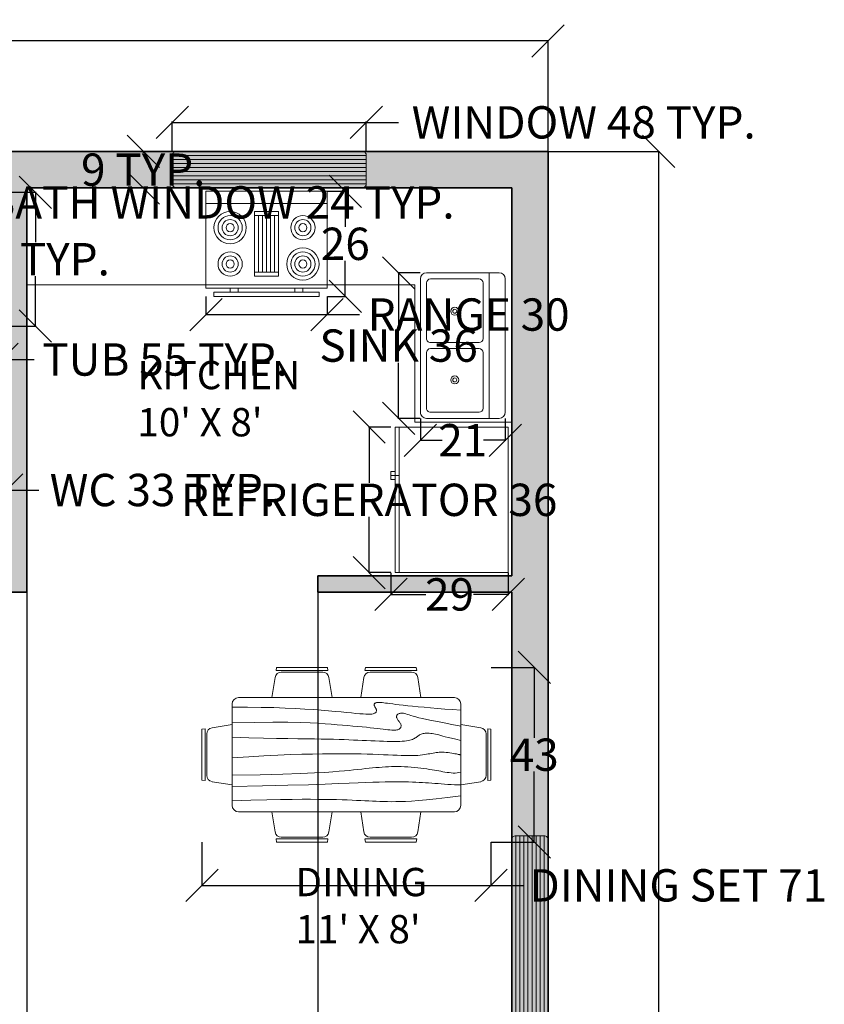
# Model space of a CAD drawing. Units: inches. Extents: x -8 to 447, y -560 to 47.
# Tile 5 of 5: x 248 to 447, y -196 to 47. Entities that reach past the tile are written whole.
import ezdxf

# ---------------------------------------------------------------- set-up
doc = ezdxf.new("R2010")
doc.units = ezdxf.units.IN
doc.header["$MEASUREMENT"] = 0
for name, color, linetype, lineweight in [('A-ANNO-DIMS', 2, 'Continuous', 18), ('A-AREA-IDEN', 7, 'Continuous', 18), ('A-EQPM', 9, 'Continuous', 18), ('A-FLOR-CASE', 8, 'Continuous', 18), ('A-FLOR-FIXT', 8, 'Continuous', 18), ('A-FURN', 8, 'Continuous', 18), ('A-WALL', 7, 'Continuous', 35), ('A-WALL-PATT', 251, 'Continuous', 13), ('WINDOW', 151, 'Continuous', 13)]:
    doc.layers.add(name, color=color, linetype=linetype, lineweight=lineweight)
doc.styles.get("Standard").update_dxf_attribs({"font": 'arial.ttf'})
doc.dimstyles.get("Standard").update_dxf_attribs({"dimtxt": 8, "dimasz": 8, "dimexe": 0.18, "dimexo": 0.0625, "dimgap": 0.09, "dimtad": 0, "dimtih": 1, "dimtoh": 1, "dimdec": 0, "dimzin": 0, "dimdsep": 46, "dimlunit": 4, "dimtxsty": 'Standard', "dimblk": 'OBLIQUE', "dimcen": 0.09, "dimadec": 0, "dimazin": 0, "dimtfac": 1, "dimtdec": 0, "dimtofl": 0, "dimtmove": 0, "dimatfit": 3, "dimldrblk": 'OBLIQUE', "dimfxl": 1, "dimtolj": 1, "dimtzin": 0, "dimarcsym": 0})

# ---------------------------------------------------------------- blocks, each defined once
blk = doc.blocks.new('WINDOW')
for p, q in [((0, -1.63), (48, -1.63)), ((0, -2.63), (48, -2.63)), ((0, -3.63), (48, -3.63)), ((0, -4.63), (48, -4.63)), ((0, -5.63), (48, -5.63)), ((0, -6.63), (48, -6.63)), ((0, -7.63), (48, -7.63)), ((0, -8.63), (48, -8.63))]:
    blk.add_line(p, q)
blk.add_lwpolyline([(48, -1.63), (48, -8.63, -0.414214), (47, -9.63), (1, -9.63, -0.414214), (0, -8.63), (0, -1.63, -0.414214), (1, -0.63), (47, -0.63, -0.414214)], format="xyb", close=True)
blk = doc.blocks.new('Dining Set - 36 x 72 in.')
for p, q in [((-22, 27.5), (-22.16, 26.5)), ((-5.84, 26.5), (-22.15, 26.5)), ((-22, 27.5), (-6, 27.5)), ((-20.52, 26), (-7.48, 26)), ((-5.84, 26.5), (-6, 27.5)), ((6, 27.5), (5.84, 26.5)), ((22.16, 26.5), (5.85, 26.5)), ((6, 27.5), (22, 27.5)), ((7.48, 26), (20.52, 26)), ((22.16, 26.5), (22, 27.5)), ((-22.5, 24.31), (-23.48, 18)), ((-4.52, 18), (-5.5, 24.31)), ((5.5, 24.31), (4.52, 18)), ((23.48, 18), (22.5, 24.31)), ((-36, 16), (-36, -16)), ((34, 18), (-34, 18)), ((36, -16), (36, 16)), ((-42.31, 8.5), (-36, 9.48)), ((42.31, 8.5), (36, 9.48)), ((-45.5, 8), (-44.5, 8.16)), ((-45.5, 8), (-45.5, -8)), ((-44.5, -8.16), (-44.5, 8.15)), ((-44, 6.52), (-44, -6.52)), ((44, 6.52), (44, -6.52)), ((45.5, 8), (44.5, 8.16)), ((44.5, -8.16), (44.5, 8.15)), ((45.5, 8), (45.5, -8)), ((-44.5, -8.16), (-45.5, -8)), ((-36, -9.48), (-42.31, -8.5)), ((36, -9.48), (42.31, -8.5)), ((44.5, -8.16), (45.5, -8)), ((-34, -18), (34, -18)), ((-22.5, -24.31), (-23.48, -18)), ((-4.52, -18), (-5.5, -24.31)), ((5.5, -24.31), (4.52, -18)), ((23.48, -18), (22.5, -24.31)), ((-22, -27.5), (-22.16, -26.5)), ((-5.84, -26.5), (-22.15, -26.5)), ((-22, -27.5), (-6, -27.5)), ((-20.52, -26), (-7.48, -26)), ((-5.84, -26.5), (-6, -27.5)), ((6, -27.5), (5.84, -26.5)), ((22.16, -26.5), (5.85, -26.5)), ((6, -27.5), (22, -27.5)), ((7.48, -26), (20.52, -26)), ((22.16, -26.5), (22, -27.5))]:
    blk.add_line(p, q)
for points in [[(-36, 15), (-31.18, 14.98), (-26.81, 14.91), (-22.85, 14.82), (-19.28, 14.69), (-16.04, 14.54), (-13.1, 14.37), (-10.42, 14.19), (-7.96, 14), (-5.69, 13.81), (-3.6, 13.63), (-1.7, 13.46), (0.04, 13.29), (1.59, 13.14), (2.98, 13.02), (4.2, 12.91), (5.25, 12.83), (6.14, 12.79), (6.88, 12.77), (7.49, 12.78), (7.98, 12.81), (8.37, 12.87), (8.67, 12.95), (8.9, 13.05), (9.08, 13.17), (9.22, 13.3), (9.32, 13.44), (9.39, 13.6), (9.43, 13.76), (9.44, 13.93), (9.42, 14.09), (9.39, 14.26), (9.33, 14.42), (9.26, 14.57), (9.18, 14.71), (9.1, 14.85), (9.01, 14.99), (8.93, 15.12), (8.85, 15.25), (8.79, 15.37), (8.75, 15.5), (8.73, 15.62), (8.73, 15.75), (8.76, 15.87), (8.81, 15.98), (8.89, 16.08), (8.98, 16.18), (9.11, 16.26), (9.25, 16.33), (9.42, 16.39), (9.62, 16.43), (9.85, 16.45), (10.12, 16.46), (10.45, 16.45), (10.82, 16.43), (11.25, 16.39), (11.75, 16.33), (12.32, 16.26), (12.97, 16.18), (13.72, 16.08), (14.57, 15.97), (15.54, 15.85), (16.64, 15.71), (17.89, 15.57), (19.29, 15.42), (20.86, 15.26), (22.59, 15.09), (24.47, 14.92), (26.51, 14.74), (28.68, 14.56), (30.99, 14.37), (33.43, 14.19), (36, 14)], [(-36, 10), (-28.98, 10.14), (-23.17, 10.2), (-18.42, 10.2), (-14.57, 10.14), (-11.44, 10.03), (-8.88, 9.89), (-6.72, 9.74), (-4.79, 9.58), (-2.97, 9.43), (-1.22, 9.29), (0.44, 9.15), (2.03, 9.01), (3.53, 8.88), (4.94, 8.75), (6.27, 8.63), (7.5, 8.5), (8.64, 8.38), (9.69, 8.25), (10.65, 8.14), (11.53, 8.03), (12.33, 7.94), (13.04, 7.86), (13.68, 7.79), (14.25, 7.75), (14.75, 7.73), (15.18, 7.73), (15.55, 7.76), (15.88, 7.8), (16.15, 7.87), (16.38, 7.95), (16.58, 8.05), (16.75, 8.17), (16.89, 8.3), (17.01, 8.45), (17.11, 8.6), (17.18, 8.77), (17.22, 8.95), (17.23, 9.13), (17.21, 9.31), (17.17, 9.5), (17.09, 9.69), (16.99, 9.88), (16.86, 10.06), (16.73, 10.25), (16.59, 10.44), (16.44, 10.62), (16.3, 10.81), (16.17, 11), (16.05, 11.19), (15.95, 11.37), (15.88, 11.56), (15.82, 11.74), (15.8, 11.92), (15.8, 12.09), (15.84, 12.26), (15.92, 12.42), (16.03, 12.57), (16.18, 12.71), (16.36, 12.83), (16.57, 12.94), (16.81, 13.02), (17.08, 13.07), (17.36, 13.1), (17.67, 13.08), (17.99, 13.03), (18.34, 12.95), (18.74, 12.83), (19.19, 12.68), (19.72, 12.51), (20.33, 12.32), (21.05, 12.1), (21.88, 11.88), (22.84, 11.63), (23.96, 11.37), (25.28, 11.09), (26.83, 10.77), (28.64, 10.4), (30.75, 9.99), (33.19, 9.53), (36, 9)], [(-36, 5.5), (-30.72, 5.33), (-26.07, 5.21), (-21.99, 5.12), (-18.43, 5.05), (-15.3, 5.01), (-12.55, 4.97), (-10.11, 4.95), (-7.92, 4.92), (-5.91, 4.88), (-4.06, 4.84), (-2.34, 4.79), (-0.74, 4.74), (0.77, 4.68), (2.22, 4.62), (3.62, 4.56), (5, 4.5), (6.37, 4.44), (7.73, 4.38), (9.07, 4.32), (10.38, 4.27), (11.63, 4.23), (12.83, 4.2), (13.96, 4.17), (15, 4.17), (15.95, 4.17), (16.82, 4.2), (17.6, 4.24), (18.3, 4.29), (18.93, 4.36), (19.49, 4.45), (19.98, 4.55), (20.42, 4.67), (20.8, 4.8), (21.13, 4.94), (21.42, 5.1), (21.69, 5.26), (21.93, 5.43), (22.15, 5.59), (22.37, 5.76), (22.58, 5.92), (22.81, 6.07), (23.04, 6.21), (23.29, 6.34), (23.55, 6.46), (23.84, 6.56), (24.14, 6.64), (24.47, 6.71), (24.83, 6.75), (25.22, 6.77), (25.64, 6.77), (26.09, 6.74), (26.55, 6.7), (27.04, 6.63), (27.54, 6.55), (28.06, 6.45), (28.58, 6.33), (29.12, 6.2), (29.71, 6.05), (30.37, 5.87), (31.14, 5.67), (32.05, 5.43), (33.14, 5.16), (34.45, 4.85), (36, 4.5)], [(-36, -1), (-30.79, -0.66), (-26.02, -0.38), (-21.65, -0.16), (-17.66, 0.01), (-14, 0.13), (-10.65, 0.21), (-7.58, 0.27), (-4.75, 0.29), (-2.13, 0.3), (0.29, 0.29), (2.53, 0.26), (4.61, 0.22), (6.55, 0.18), (8.36, 0.12), (10.06, 0.06), (11.67, 0), (13.19, -0.06), (14.63, -0.12), (16, -0.17), (17.28, -0.22), (18.48, -0.25), (19.6, -0.27), (20.63, -0.27), (21.58, -0.25), (22.45, -0.21), (23.24, -0.15), (23.95, -0.07), (24.61, 0.02), (25.22, 0.12), (25.79, 0.22), (26.32, 0.32), (26.83, 0.42), (27.33, 0.51), (27.81, 0.59), (28.29, 0.65), (28.77, 0.71), (29.26, 0.75), (29.76, 0.77), (30.29, 0.77), (30.83, 0.75), (31.41, 0.71), (32, 0.65), (32.59, 0.57), (33.16, 0.49), (33.7, 0.4), (34.19, 0.32), (34.62, 0.24), (34.96, 0.17), (35.21, 0.11), (35.38, 0.07), (35.5, 0.04), (35.59, 0.02), (35.66, 0.01), (35.74, 0), (35.84, 0), (36, 0)], [(-36, -6.5), (-27.18, -6.31), (-20.08, -6.13), (-14.47, -5.94), (-10.11, -5.76), (-6.78, -5.58), (-4.24, -5.41), (-2.26, -5.24), (-0.62, -5.08), (0.87, -4.93), (2.27, -4.79), (3.59, -4.65), (4.83, -4.52), (6, -4.4), (7.13, -4.29), (8.21, -4.18), (9.25, -4.08), (10.27, -3.99), (11.27, -3.91), (12.26, -3.85), (13.25, -3.79), (14.24, -3.75), (15.23, -3.73), (16.23, -3.73), (17.25, -3.75), (18.29, -3.79), (19.35, -3.86), (20.4, -3.94), (21.45, -4.03), (22.48, -4.14), (23.47, -4.25), (24.43, -4.38), (25.33, -4.5), (26.18, -4.62), (26.97, -4.75), (27.71, -4.87), (28.42, -4.99), (29.1, -5.11), (29.76, -5.23), (30.4, -5.35), (31.04, -5.46), (31.68, -5.56), (32.33, -5.66), (32.97, -5.73), (33.6, -5.78), (34.22, -5.78), (34.83, -5.75), (35.43, -5.65), (36, -5.5)], [(-36, -10), (-26.4, -9.81), (-18.47, -9.63), (-11.98, -9.45), (-6.74, -9.28), (-2.52, -9.12), (0.88, -8.98), (3.68, -8.85), (6.08, -8.75), (8.28, -8.67), (10.3, -8.61), (12.17, -8.57), (13.9, -8.54), (15.49, -8.53), (16.96, -8.54), (18.32, -8.56), (19.58, -8.58), (20.76, -8.62), (21.87, -8.66), (22.92, -8.71), (23.93, -8.77), (24.91, -8.83), (25.88, -8.89), (26.85, -8.97), (27.83, -9.04), (28.85, -9.12), (29.88, -9.2), (30.93, -9.28), (31.98, -9.35), (33.02, -9.41), (34.04, -9.46), (35.04, -9.49), (36, -9.5)], [(-36, -14.5), (-30.09, -14.34), (-25.03, -14.21), (-20.73, -14.13), (-17.08, -14.07), (-13.97, -14.05), (-11.3, -14.04), (-8.97, -14.06), (-6.88, -14.08), (-4.92, -14.12), (-3.09, -14.16), (-1.37, -14.21), (0.24, -14.26), (1.76, -14.32), (3.2, -14.38), (4.55, -14.44), (5.83, -14.5), (7.06, -14.56), (8.24, -14.62), (9.39, -14.68), (10.55, -14.72), (11.72, -14.76), (12.93, -14.79), (14.2, -14.8), (15.54, -14.79), (16.99, -14.76), (18.62, -14.71), (20.48, -14.6), (22.66, -14.44), (25.23, -14.22), (28.26, -13.91), (31.83, -13.51), (36, -13)]]:
    blk.add_lwpolyline(points)
for centre, start, end in [((-20.52, 24), 90, 171.1198), ((-7.48, 24), 8.881, 90), ((7.48, 24), 90, 171.1198), ((20.52, 24), 8.881, 90), ((-34, 16), 90, 180), ((34, 16), 0, 90), ((-42, 6.52), 98.8806, 180), ((42, 6.52), 0, 81.1194), ((-42, -6.52), 180, 261.1194), ((42, -6.52), 278.8806, 0), ((-34, -16), 180, 270), ((34, -16), 270, 0), ((-20.52, -24), 188.8802, 270), ((-7.48, -24), 270, 351.1191), ((7.48, -24), 188.8802, 270), ((20.52, -24), 270, 351.1191)]:
    blk.add_arc(centre, 2, start, end)
blk = doc.blocks.new('Range-Oven - 30 in top')
for p, q in [((0, -3), (30, -3)), ((12, -6), (18, -6)), ((13, -20), (13, -6)), ((14, -6), (14, -20)), ((15, -20), (15, -6)), ((16, -6), (16, -20)), ((17, -20), (17, -6)), ((18, -20), (12, -20)), ((6, -24), (6, -25)), ((8, -25), (8, -24)), ((22, -25), (22, -24)), ((24, -24), (24, -25))]:
    blk.add_line(p, q)
for points in [[(0, -24), (0, 0), (30, 0), (30, -24)], [(12, -21), (12, -5), (18, -5), (18, -21)], [(2, -26), (2, -25), (28, -25), (28, -26)]]:
    blk.add_lwpolyline(points, close=True)
for centre, radius in [((6, -9), 4), ((6, -9), 3), ((6, -9), 2), ((24, -9), 3), ((24, -9), 2), ((6, -9), 1), ((24, -9), 1), ((24, -18), 4), ((6, -18), 3), ((6, -18), 2), ((6, -18), 1), ((24, -18), 3), ((24, -18), 2), ((24, -18), 1)]:
    blk.add_circle(centre, radius)
blk = doc.blocks.new('Sink-double - 36 in top')
for p, q in [((-18, -4), (18, -4)), ((-0.75, -18.5), (-0.75, -6.5)), ((0.75, -6.5), (0.75, -18.5))]:
    blk.add_line(p, q)
for points in [[(-16.5, 0), (16.5, 0)], [(-18, -19.5), (-18, -1.5)], [(18, -1.5), (18, -19.5)], [(-16.5, -18.5), (-16.5, -6.5)], [(-15.5, -5.5), (-1.75, -5.5)], [(1.75, -5.5), (15.5, -5.5)], [(16.5, -6.5), (16.5, -18.5)], [(16.5, -21), (-16.5, -21)], [(-1.75, -19.5), (-15.5, -19.5)], [(15.5, -19.5), (1.75, -19.5)]]:
    blk.add_lwpolyline(points)
for centre, radius in [((-8.5, -12.5), 1), ((-8.5, -12.5), 0.5), ((8.5, -12.5), 1), ((8.5, -12.5), 0.5)]:
    blk.add_circle(centre, radius)
for centre, radius, start, end in [((-16.5, -1.5), 1.5, 90, 180), ((16.5, -1.5), 1.5, 0, 90), ((-15.5, -6.5), 1, 90, 180), ((-1.75, -6.5), 1, 0, 90), ((1.75, -6.5), 1, 90, 180), ((15.5, -6.5), 1, 0, 90), ((-15.5, -18.5), 1, 180, 270), ((-1.75, -18.5), 1, 270, 0), ((1.75, -18.5), 1, 180, 270), ((15.5, -18.5), 1, 270, 0), ((-16.5, -19.5), 1.5, 180, 270), ((16.5, -19.5), 1.5, 270, 0)]:
    blk.add_arc(centre, radius, start, end)
blk = doc.blocks.new('Refrigerator-2 door - 36 in top')
for p, q in [((0, -26.999999), (36, -26.999999)), ((11, -27.999999), (11, -28.999999)), ((11, -28.999999), (13, -28.999999)), ((12, -26.999999), (12, -28.999999)), ((13, -28.999999), (13, -27.999999))]:
    blk.add_line(p, q)
blk.add_lwpolyline([(0, -27.999999), (0, 0), (36, 0), (36, -27.999999)], close=True)
blk = doc.blocks.new('_Oblique')
at = {"color": 0, "linetype": 'ByBlock', "lineweight": -2}
blk.add_line((-0.5, -0.5), (0.5, 0.5), dxfattribs=at)
blk = doc.blocks.new('*D29')
at = {"layer": 'A-ANNO-DIMS', "color": 0, "lineweight": -2, "transparency": 16777216}
for p, q in [((285.7, 14.62), (285.7, 21.94)), ((333.7, 14.62), (333.7, 21.94)), ((285.7, 21.76), (333.7, 21.76)), ((333.7, 21.76), (341.7, 21.76))]:
    blk.add_line(p, q, dxfattribs=at)
at = {"layer": 'Defpoints', "color": 0, "transparency": 16777216}
for p in [(333.7, 21.76), (285.7, 14.56), (333.7, 14.56)]:
    blk.add_point(p, dxfattribs=at)
at = {"layer": 'A-ANNO-DIMS', "color": 0, "lineweight": -2, "transparency": 16777216, "xscale": 8, "yscale": 8, "zscale": 8, "rotation": 180}
blk.add_blockref('_Oblique', (285.7, 21.76), dxfattribs=at)
at = {"layer": 'A-ANNO-DIMS', "color": 0, "lineweight": -2, "transparency": 16777216, "xscale": 8, "yscale": 8, "zscale": 8}
blk.add_blockref('_Oblique', (333.7, 21.76), dxfattribs=at)
at = {"layer": 'A-ANNO-DIMS', "color": 0, "transparency": 16777216, "insert": (387.5, 21.76), "char_height": 8, "attachment_point": 5}
blk.add_mtext('\\A1;WINDOW 48 TYP.', dxfattribs=at)
blk = doc.blocks.new('*D30')
at = {"layer": 'A-ANNO-DIMS', "color": 0, "lineweight": -2, "transparency": 16777216}
for p, q in [((285.64, 14.56), (278.32, 14.56)), ((278.5, 14.56), (278.5, 14.23)), ((285.64, 5.56), (278.32, 5.56)), ((278.5, 5.56), (278.5, 5.89))]:
    blk.add_line(p, q, dxfattribs=at)
at = {"layer": 'Defpoints', "color": 0, "transparency": 16777216}
for p in [(278.5, 14.56), (285.7, 14.56), (285.7, 5.56)]:
    blk.add_point(p, dxfattribs=at)
at = {"layer": 'A-ANNO-DIMS', "color": 0, "lineweight": -2, "transparency": 16777216, "xscale": 8, "yscale": 8, "zscale": 8}
for p, rotation in [((278.5, 14.56), 90), ((278.5, 5.56), 270)]:
    blk.add_blockref('_Oblique', p, dxfattribs=dict(at, rotation=rotation))
at = {"layer": 'A-ANNO-DIMS', "color": 0, "transparency": 16777216, "insert": (278.5, 10.06), "char_height": 8, "attachment_point": 5}
blk.add_mtext('\\A1;9 TYP.', dxfattribs=at)
blk = doc.blocks.new('*D31')
at = {"layer": 'A-ANNO-DIMS', "color": 0, "lineweight": -2, "transparency": 16777216}
for p, q in [((203.7, 5.5), (203.7, 1.78)), ((227.7, 5.5), (227.7, 1.78)), ((203.7, 1.96), (227.7, 1.96)), ((227.7, 1.96), (235.7, 1.96))]:
    blk.add_line(p, q, dxfattribs=at)
at = {"layer": 'Defpoints', "color": 0, "transparency": 16777216}
for p in [(203.7, 5.56), (227.7, 5.56), (227.7, 1.96)]:
    blk.add_point(p, dxfattribs=at)
at = {"layer": 'A-ANNO-DIMS', "color": 0, "lineweight": -2, "transparency": 16777216, "xscale": 8, "yscale": 8, "zscale": 8, "rotation": 180}
blk.add_blockref('_Oblique', (203.7, 1.96), dxfattribs=at)
at = {"layer": 'A-ANNO-DIMS', "color": 0, "lineweight": -2, "transparency": 16777216, "xscale": 8, "yscale": 8, "zscale": 8}
blk.add_blockref('_Oblique', (227.7, 1.96), dxfattribs=at)
at = {"layer": 'A-ANNO-DIMS', "color": 0, "transparency": 16777216, "insert": (297.61, 1.96), "char_height": 8, "attachment_point": 5}
blk.add_mtext('\\A1;BATH WINDOW 24 TYP.', dxfattribs=at)
blk = doc.blocks.new('*D39')
at = {"layer": 'A-ANNO-DIMS', "color": 0, "lineweight": -2, "transparency": 16777216}
for p, q in [((211.63, -64.31), (211.63, -69.38)), ((244.67, -64.31), (244.67, -69.38)), ((211.63, -69.2), (244.67, -69.2)), ((244.67, -69.2), (252.67, -69.2))]:
    blk.add_line(p, q, dxfattribs=at)
at = {"layer": 'Defpoints', "color": 0, "transparency": 16777216}
for p in [(211.63, -64.25), (244.67, -64.25), (244.67, -69.2)]:
    blk.add_point(p, dxfattribs=at)
at = {"layer": 'A-ANNO-DIMS', "color": 0, "lineweight": -2, "transparency": 16777216, "xscale": 8, "yscale": 8, "zscale": 8, "rotation": 180}
blk.add_blockref('_Oblique', (211.63, -69.2), dxfattribs=at)
at = {"layer": 'A-ANNO-DIMS', "color": 0, "lineweight": -2, "transparency": 16777216, "xscale": 8, "yscale": 8, "zscale": 8}
blk.add_blockref('_Oblique', (244.67, -69.2), dxfattribs=at)
at = {"layer": 'A-ANNO-DIMS', "color": 0, "transparency": 16777216, "insert": (283.26, -69.2), "char_height": 8, "attachment_point": 5}
blk.add_mtext('\\A1;WC 33 TYP.', dxfattribs=at)
blk = doc.blocks.new('*D41')
at = {"layer": 'A-ANNO-DIMS', "color": 0, "lineweight": -2, "transparency": 16777216}
for p, q in [((188.4, -28.7), (188.4, -37.09)), ((243.54, -28.7), (243.54, -37.09)), ((188.4, -36.91), (243.54, -36.91)), ((243.54, -36.91), (251.54, -36.91))]:
    blk.add_line(p, q, dxfattribs=at)
at = {"layer": 'Defpoints', "color": 0, "transparency": 16777216}
for p in [(188.4, -28.64), (243.54, -28.64), (243.54, -36.91)]:
    blk.add_point(p, dxfattribs=at)
at = {"layer": 'A-ANNO-DIMS', "color": 0, "lineweight": -2, "transparency": 16777216, "xscale": 8, "yscale": 8, "zscale": 8, "rotation": 180}
blk.add_blockref('_Oblique', (188.4, -36.91), dxfattribs=at)
at = {"layer": 'A-ANNO-DIMS', "color": 0, "lineweight": -2, "transparency": 16777216, "xscale": 8, "yscale": 8, "zscale": 8}
blk.add_blockref('_Oblique', (243.54, -36.91), dxfattribs=at)
at = {"layer": 'A-ANNO-DIMS', "color": 0, "transparency": 16777216, "insert": (283.93, -36.91), "char_height": 8, "attachment_point": 5}
blk.add_mtext('\\A1;TUB 55 TYP.', dxfattribs=at)
blk = doc.blocks.new('*D42')
at = {"layer": 'A-ANNO-DIMS', "color": 0, "lineweight": -2, "transparency": 16777216}
for p, q in [((243.61, 4.45), (252, 4.45)), ((251.82, 4.45), (251.82, -7.92)), ((251.82, -28.64), (251.82, -16.28)), ((243.61, -28.64), (252, -28.64))]:
    blk.add_line(p, q, dxfattribs=at)
at = {"layer": 'Defpoints', "color": 0, "transparency": 16777216}
for p in [(243.54, 4.45), (251.82, 4.45), (243.54, -28.64)]:
    blk.add_point(p, dxfattribs=at)
at = {"layer": 'A-ANNO-DIMS', "color": 0, "lineweight": -2, "transparency": 16777216, "xscale": 8, "yscale": 8, "zscale": 8}
for p, rotation in [((251.82, 4.45), 90), ((251.82, -28.64), 270)]:
    blk.add_blockref('_Oblique', p, dxfattribs=dict(at, rotation=rotation))
at = {"layer": 'A-ANNO-DIMS', "color": 0, "transparency": 16777216, "insert": (251.82, -12.1), "char_height": 8, "attachment_point": 5}
blk.add_mtext('\\A1;33 TYP.', dxfattribs=at)
blk = doc.blocks.new('*D43')
at = {"layer": 'A-ANNO-DIMS', "color": 0, "lineweight": -2, "transparency": 16777216}
for p, q in [((293.04, -156.35), (293.04, -167.19)), ((364.53, -156.35), (364.53, -167.19)), ((293.04, -167.01), (364.53, -167.01)), ((364.53, -167.01), (372.53, -167.01))]:
    blk.add_line(p, q, dxfattribs=at)
at = {"layer": 'Defpoints', "color": 0, "transparency": 16777216}
for p in [(293.04, -156.29), (364.53, -156.29), (364.53, -167.01)]:
    blk.add_point(p, dxfattribs=at)
at = {"layer": 'A-ANNO-DIMS', "color": 0, "lineweight": -2, "transparency": 16777216, "xscale": 8, "yscale": 8, "zscale": 8, "rotation": 180}
blk.add_blockref('_Oblique', (293.04, -167.01), dxfattribs=at)
at = {"layer": 'A-ANNO-DIMS', "color": 0, "lineweight": -2, "transparency": 16777216, "xscale": 8, "yscale": 8, "zscale": 8}
blk.add_blockref('_Oblique', (364.53, -167.01), dxfattribs=at)
at = {"layer": 'A-ANNO-DIMS', "color": 0, "transparency": 16777216, "insert": (410.91, -167.01), "char_height": 8, "attachment_point": 5}
blk.add_mtext('\\A1;DINING SET 71', dxfattribs=at)
blk = doc.blocks.new('*D44')
at = {"layer": 'A-ANNO-DIMS', "color": 0, "lineweight": -2, "transparency": 16777216}
for p, q in [((364.59, -113.08), (375.44, -113.08)), ((375.26, -113.08), (375.26, -130.5)), ((375.26, -156.29), (375.26, -138.86)), ((364.59, -156.29), (375.44, -156.29))]:
    blk.add_line(p, q, dxfattribs=at)
at = {"layer": 'Defpoints', "color": 0, "transparency": 16777216}
for p in [(364.53, -113.08), (375.26, -113.08), (364.53, -156.29)]:
    blk.add_point(p, dxfattribs=at)
at = {"layer": 'A-ANNO-DIMS', "color": 0, "lineweight": -2, "transparency": 16777216, "xscale": 8, "yscale": 8, "zscale": 8}
for p, rotation in [((375.26, -113.08), 90), ((375.26, -156.29), 270)]:
    blk.add_blockref('_Oblique', p, dxfattribs=dict(at, rotation=rotation))
at = {"layer": 'A-ANNO-DIMS', "color": 0, "transparency": 16777216, "insert": (375.26, -134.68), "char_height": 8, "attachment_point": 5}
blk.add_mtext('\\A1;43', dxfattribs=at)
blk = doc.blocks.new('*D45')
at = {"layer": 'A-ANNO-DIMS', "color": 0, "lineweight": -2, "transparency": 16777216}
for p, q in [((294.01, -21.35), (294.01, -25.97)), ((324.01, -21.35), (324.01, -25.97)), ((294.01, -25.79), (324.01, -25.79)), ((324.01, -25.79), (332.01, -25.79))]:
    blk.add_line(p, q, dxfattribs=at)
at = {"layer": 'Defpoints', "color": 0, "transparency": 16777216}
for p in [(294.01, -21.29), (324.01, -21.29), (324.01, -25.79)]:
    blk.add_point(p, dxfattribs=at)
at = {"layer": 'A-ANNO-DIMS', "color": 0, "lineweight": -2, "transparency": 16777216, "xscale": 8, "yscale": 8, "zscale": 8, "rotation": 180}
blk.add_blockref('_Oblique', (294.01, -25.79), dxfattribs=at)
at = {"layer": 'A-ANNO-DIMS', "color": 0, "lineweight": -2, "transparency": 16777216, "xscale": 8, "yscale": 8, "zscale": 8}
blk.add_blockref('_Oblique', (324.01, -25.79), dxfattribs=at)
at = {"layer": 'A-ANNO-DIMS', "color": 0, "transparency": 16777216, "insert": (359.03, -25.79), "char_height": 8, "attachment_point": 5}
blk.add_mtext('\\A1;RANGE 30', dxfattribs=at)
blk = doc.blocks.new('*D46')
at = {"layer": 'A-ANNO-DIMS', "color": 0, "lineweight": -2, "transparency": 16777216}
for p, q in [((324.07, 4.71), (328.69, 4.71)), ((328.51, 4.71), (328.51, -4.11)), ((328.51, -21.29), (328.51, -12.46)), ((324.07, -21.29), (328.69, -21.29))]:
    blk.add_line(p, q, dxfattribs=at)
at = {"layer": 'Defpoints', "color": 0, "transparency": 16777216}
for p in [(324.01, 4.71), (328.51, 4.71), (324.01, -21.29)]:
    blk.add_point(p, dxfattribs=at)
at = {"layer": 'A-ANNO-DIMS', "color": 0, "lineweight": -2, "transparency": 16777216, "xscale": 8, "yscale": 8, "zscale": 8}
for p, rotation in [((328.51, 4.71), 90), ((328.51, -21.29), 270)]:
    blk.add_blockref('_Oblique', p, dxfattribs=dict(at, rotation=rotation))
at = {"layer": 'A-ANNO-DIMS', "color": 0, "transparency": 16777216, "insert": (328.51, -8.29), "char_height": 8, "attachment_point": 5}
blk.add_mtext('\\A1;26', dxfattribs=at)
blk = doc.blocks.new('*D47')
at = {"layer": 'A-ANNO-DIMS', "color": 0, "lineweight": -2, "transparency": 16777216}
for p, q in [((347.03, -15.47), (341.51, -15.47)), ((341.69, -15.47), (341.69, -29.24)), ((341.69, -51.47), (341.69, -37.7)), ((347.03, -51.47), (341.51, -51.47))]:
    blk.add_line(p, q, dxfattribs=at)
at = {"layer": 'Defpoints', "color": 0, "transparency": 16777216}
for p in [(347.09, -15.47), (341.69, -51.47), (347.09, -51.47)]:
    blk.add_point(p, dxfattribs=at)
at = {"layer": 'A-ANNO-DIMS', "color": 0, "lineweight": -2, "transparency": 16777216, "xscale": 8, "yscale": 8, "zscale": 8}
for p, rotation in [((341.69, -15.47), 90), ((341.69, -51.47), 270)]:
    blk.add_blockref('_Oblique', p, dxfattribs=dict(at, rotation=rotation))
at = {"layer": 'A-ANNO-DIMS', "color": 0, "transparency": 16777216, "insert": (341.69, -33.47), "char_height": 8, "attachment_point": 5}
blk.add_mtext('\\A1;SINK 36', dxfattribs=at)
blk = doc.blocks.new('*D48')
at = {"layer": 'A-ANNO-DIMS', "color": 0, "lineweight": -2, "transparency": 16777216}
for p, q in [((347.09, -51.53), (347.09, -57.05)), ((368.09, -51.53), (368.09, -57.05)), ((347.09, -56.87), (352.48, -56.87)), ((368.09, -56.87), (362.71, -56.87))]:
    blk.add_line(p, q, dxfattribs=at)
at = {"layer": 'Defpoints', "color": 0, "transparency": 16777216}
for p in [(347.09, -51.47), (368.09, -51.47), (368.09, -56.87)]:
    blk.add_point(p, dxfattribs=at)
at = {"layer": 'A-ANNO-DIMS', "color": 0, "lineweight": -2, "transparency": 16777216, "xscale": 8, "yscale": 8, "zscale": 8, "rotation": 180}
blk.add_blockref('_Oblique', (347.09, -56.87), dxfattribs=at)
at = {"layer": 'A-ANNO-DIMS', "color": 0, "lineweight": -2, "transparency": 16777216, "xscale": 8, "yscale": 8, "zscale": 8}
blk.add_blockref('_Oblique', (368.09, -56.87), dxfattribs=at)
at = {"layer": 'A-ANNO-DIMS', "color": 0, "transparency": 16777216, "insert": (357.59, -56.87), "char_height": 8, "attachment_point": 5}
blk.add_mtext('\\A1;21', dxfattribs=at)
blk = doc.blocks.new('*D49')
at = {"layer": 'A-ANNO-DIMS', "color": 0, "lineweight": -2, "transparency": 16777216}
for p, q in [((339.74, -53.63), (334.23, -53.63)), ((334.41, -53.63), (334.41, -67.4)), ((334.41, -89.63), (334.41, -75.86)), ((339.74, -89.63), (334.23, -89.63))]:
    blk.add_line(p, q, dxfattribs=at)
at = {"layer": 'Defpoints', "color": 0, "transparency": 16777216}
for p in [(339.81, -53.63), (334.41, -89.63), (339.81, -89.63)]:
    blk.add_point(p, dxfattribs=at)
at = {"layer": 'A-ANNO-DIMS', "color": 0, "lineweight": -2, "transparency": 16777216, "xscale": 8, "yscale": 8, "zscale": 8}
for p, rotation in [((334.41, -53.63), 90), ((334.41, -89.63), 270)]:
    blk.add_blockref('_Oblique', p, dxfattribs=dict(at, rotation=rotation))
at = {"layer": 'A-ANNO-DIMS', "color": 0, "transparency": 16777216, "insert": (334.41, -71.63), "char_height": 8, "attachment_point": 5}
blk.add_mtext('\\A1;REFRIGERATOR 36', dxfattribs=at)
blk = doc.blocks.new('*D50')
at = {"layer": 'A-ANNO-DIMS', "color": 0, "lineweight": -2, "transparency": 16777216}
for p, q in [((339.81, -89.69), (339.81, -95.21)), ((368.81, -89.69), (368.81, -95.21)), ((339.81, -95.03), (348.41, -95.03)), ((368.81, -95.03), (360.2, -95.03))]:
    blk.add_line(p, q, dxfattribs=at)
at = {"layer": 'Defpoints', "color": 0, "transparency": 16777216}
for p in [(339.81, -89.63), (368.81, -89.63), (368.81, -95.03)]:
    blk.add_point(p, dxfattribs=at)
at = {"layer": 'A-ANNO-DIMS', "color": 0, "lineweight": -2, "transparency": 16777216, "xscale": 8, "yscale": 8, "zscale": 8, "rotation": 180}
blk.add_blockref('_Oblique', (339.81, -95.03), dxfattribs=at)
at = {"layer": 'A-ANNO-DIMS', "color": 0, "lineweight": -2, "transparency": 16777216, "xscale": 8, "yscale": 8, "zscale": 8}
blk.add_blockref('_Oblique', (368.81, -95.03), dxfattribs=at)
at = {"layer": 'A-ANNO-DIMS', "color": 0, "transparency": 16777216, "insert": (354.31, -95.03), "char_height": 8, "attachment_point": 5}
blk.add_mtext('\\A1;29', dxfattribs=at)
blk = doc.blocks.new('*D51')
at = {"layer": 'A-ANNO-DIMS', "color": 0, "lineweight": -2, "transparency": 16777216}
for p, q in [((28.7, 14.62), (28.7, 42.09)), ((28.7, 41.91), (194.79, 41.91)), ((378.7, 41.91), (212.61, 41.91)), ((378.7, 14.62), (378.7, 42.09))]:
    blk.add_line(p, q, dxfattribs=at)
at = {"layer": 'Defpoints', "color": 0, "transparency": 16777216}
for p in [(378.7, 41.91), (28.7, 14.56), (378.7, 14.56)]:
    blk.add_point(p, dxfattribs=at)
at = {"layer": 'A-ANNO-DIMS', "color": 0, "lineweight": -2, "transparency": 16777216, "xscale": 8, "yscale": 8, "zscale": 8, "rotation": 180}
blk.add_blockref('_Oblique', (28.7, 41.91), dxfattribs=at)
at = {"layer": 'A-ANNO-DIMS', "color": 0, "lineweight": -2, "transparency": 16777216, "xscale": 8, "yscale": 8, "zscale": 8}
blk.add_blockref('_Oblique', (378.7, 41.91), dxfattribs=at)
at = {"layer": 'A-ANNO-DIMS', "color": 0, "transparency": 16777216, "insert": (203.7, 41.91), "char_height": 8, "attachment_point": 5}
blk.add_mtext('\\A1;350', dxfattribs=at)
blk = doc.blocks.new('*D52')
at = {"layer": 'A-ANNO-DIMS', "color": 0, "lineweight": -2, "transparency": 16777216}
for p, q in [((378.76, 14.56), (406.23, 14.56)), ((406.05, 14.56), (406.05, -252.27)), ((406.05, -527.44), (406.05, -260.61)), ((307.76, -527.44), (406.23, -527.44))]:
    blk.add_line(p, q, dxfattribs=at)
at = {"layer": 'Defpoints', "color": 0, "transparency": 16777216}
for p in [(378.7, 14.56), (307.7, -527.44), (406.05, -527.44)]:
    blk.add_point(p, dxfattribs=at)
at = {"layer": 'A-ANNO-DIMS', "color": 0, "lineweight": -2, "transparency": 16777216, "xscale": 8, "yscale": 8, "zscale": 8}
for p, rotation in [((406.05, 14.56), 90), ((406.05, -527.44), 270)]:
    blk.add_blockref('_Oblique', p, dxfattribs=dict(at, rotation=rotation))
at = {"layer": 'A-ANNO-DIMS', "color": 0, "transparency": 16777216, "insert": (406.05, -256.44), "char_height": 8, "attachment_point": 5}
blk.add_mtext('\\A1;542', dxfattribs=at)
blk = doc.blocks.new('*D63')
at = {"layer": 'A-ANNO-DIMS', "color": 0, "lineweight": -2, "transparency": 16777216}
for p, q in [((249.7, -94.5), (249.7, -554.97)), ((321.7, -94.5), (321.7, -554.97)), ((249.7, -554.79), (279.96, -554.79)), ((321.7, -554.79), (291.45, -554.79))]:
    blk.add_line(p, q, dxfattribs=at)
at = {"layer": 'Defpoints', "color": 0, "transparency": 16777216}
for p in [(249.7, -94.44), (321.7, -94.44), (321.7, -554.79)]:
    blk.add_point(p, dxfattribs=at)
at = {"layer": 'A-ANNO-DIMS', "color": 0, "lineweight": -2, "transparency": 16777216, "xscale": 8, "yscale": 8, "zscale": 8, "rotation": 180}
blk.add_blockref('_Oblique', (249.7, -554.79), dxfattribs=at)
at = {"layer": 'A-ANNO-DIMS', "color": 0, "lineweight": -2, "transparency": 16777216, "xscale": 8, "yscale": 8, "zscale": 8}
blk.add_blockref('_Oblique', (321.7, -554.79), dxfattribs=at)
at = {"layer": 'A-ANNO-DIMS', "color": 0, "transparency": 16777216, "insert": (285.7, -554.79), "char_height": 8, "attachment_point": 5}
blk.add_mtext('\\A1;72', dxfattribs=at)

msp = doc.modelspace()

# ---------------------------------------------------------------- hatches: boundary and pattern name
at = {"layer": 'A-WALL-PATT'}
h = msp.add_hatch(color=256, dxfattribs=at)
h.dxf.hatch_style = 1
h.paths.add_polyline_path([(378.702, 14.56), (333.702, 14.56), (333.702, 5.56), (369.702, 5.56), (369.702, -90.44), (321.702, -90.44), (321.702, -94.44), (369.702, -94.44), (369.702, -154.733), (378.702, -154.733)])
h.paths.add_polyline_path([(285.702, 14.56), (227.702, 14.56), (227.702, 5.56), (245.702, 5.56), (245.702, -90.44), (239.702, -90.44), (239.702, -94.44), (249.702, -94.44), (249.702, -90.44), (249.702, 5.56), (285.702, 5.56)])
h.paths.add_polyline_path([(203.702, 14.56), (133.702, 14.56), (133.702, 5.56), (181.702, 5.56), (181.702, -132.44), (175.702, -132.44), (175.702, -136.44), (185.702, -136.44), (185.702, -94.44), (209.702, -94.44), (209.702, -90.44), (185.702, -90.44), (185.702, 5.56), (203.702, 5.56)])
h = msp.add_hatch(color=256, dxfattribs=at)
h.dxf.hatch_style = 1
h.paths.add_polyline_path([(378.702, 14.56), (227.702, 14.56), (227.702, 5.56), (245.702, 5.56), (245.702, -90.44), (239.702, -90.44), (239.702, -94.44), (249.702, -94.44), (249.702, -90.44), (249.702, 5.56), (369.702, 5.56), (369.702, -90.44), (321.702, -90.44), (321.702, -94.44), (369.702, -94.44), (369.702, -452.44), (325.702, -452.44), (325.702, -456.44), (369.702, -456.44), (369.702, -500.44), (309.702, -500.44), (309.702, -509.44), (369.702, -509.44), (369.702, -525.44), (378.702, -525.44)])

# ---------------------------------------------------------------- linework, layer by layer
at = {"layer": 'A-FLOR-CASE'}
for p, q in [((249.702, -18.44), (345.702, -18.44)), ((345.702, -18.44), (345.702, -52.44)), ((345.702, -52.44), (345.702, -18.44)), ((345.702, -52.44), (369.702, -52.44))]:
    msp.add_line(p, q, dxfattribs=at)
at = {"layer": 'A-WALL'}
for p, q in [((28.702, 14.56), (378.702, 14.56)), ((378.702, 14.56), (378.702, -525.44)), ((249.702, 5.56), (369.702, 5.56)), ((249.702, -90.44), (249.702, 5.56)), ((369.702, 5.56), (369.702, -90.44)), ((369.702, -90.44), (369.702, 5.56)), ((249.702, -90.44), (249.702, -94.44)), ((321.702, -90.44), (369.702, -90.44)), ((321.702, -90.44), (321.702, -94.44)), ((239.702, -94.44), (249.702, -94.44)), ((321.702, -94.44), (369.702, -94.44)), ((369.702, -94.44), (369.702, -452.44))]:
    msp.add_line(p, q, dxfattribs=at)

# ---------------------------------------------------------------- block references
at = {"layer": 'A-EQPM'}
msp.add_blockref('Range-Oven - 30 in top', (294.008, 4.71), dxfattribs=at)
at = {"layer": 'A-EQPM', "rotation": 270}
msp.add_blockref('Refrigerator-2 door - 36 in top', (368.807, -53.63), dxfattribs=at)
at = {"layer": 'A-FLOR-FIXT', "rotation": 270}
msp.add_blockref('Sink-double - 36 in top', (368.095, -33.468), dxfattribs=at)
at = {"layer": 'A-FURN', "xscale": 0.7856607656645134, "yscale": 0.7856607656645134, "zscale": 0.7856607656645134}
msp.add_blockref('Dining Set - 36 x 72 in.', (328.784, -134.682), dxfattribs=at)
at = {"layer": 'WINDOW'}
msp.add_blockref('WINDOW', (285.702, 15.195), dxfattribs=at)
at = {"layer": 'WINDOW', "rotation": 270}
msp.add_blockref('WINDOW', (379.337, -154.733), dxfattribs=at)

# ---------------------------------------------------------------- texts
at = {"layer": 'A-AREA-IDEN', "char_height": 7, "attachment_point": 1}
for s, width, insert in [("KITCHEN\\P10' X 8'", 101.37701, (277.064, -37.257)), ("DINING\\P11' X 8'", 131.16623, (316.19, -162.691))]:
    msp.add_mtext_dynamic_manual_height_columns(s, width=width, gutter_width=1, heights=[0], dxfattribs=dict(at, insert=insert))

# ---------------------------------------------------------------- dimensions: what is measured, and where the dimension line sits
at = {"layer": 'A-ANNO-DIMS'}
for base, p1, p2, picture, middle in [((378.702, 41.91), (28.702, 14.56), (378.702, 14.56), '*D51', (203.702, 41.91)), ((368.095, -56.868), (347.095, -51.468), (368.095, -51.468), '*D48', (357.595, -56.868)), ((368.807, -95.03), (339.807, -89.63), (368.807, -89.63), '*D50', (354.307, -95.03)), ((321.702, -554.79), (249.702, -94.44), (321.702, -94.44), '*D63', (285.702, -554.79))]:
    dim = msp.add_linear_dim(base=base, p1=p1, p2=p2, dimstyle='Standard', override={"dimdec": 0, "dimlfac": 1, "dimrnd": 0, "dimzin": 0, "dimdsep": 46, "dimlunit": 2}, dxfattribs=at)
    dim.commit()
    dim.dimension.update_dxf_attribs({"geometry": picture, "text_midpoint": middle})
for base, p1, p2, text, picture, middle in [((333.702, 21.76), (285.702, 14.56), (333.702, 14.56), 'WINDOW <> TYP.', '*D29', (387.498, 21.76)), ((227.702, 1.96), (203.702, 5.56), (227.702, 5.56), 'BATH WINDOW <> TYP.', '*D31', (297.612, 1.96)), ((324.008, -25.79), (294.008, -21.29), (324.008, -21.29), 'RANGE <>', '*D45', (359.031, -25.79)), ((243.545, -36.914), (188.397, -28.642), (243.545, -28.642), 'TUB <> TYP.', '*D41', (283.935, -36.914)), ((244.672, -69.204), (211.626, -64.247), (244.672, -64.247), 'WC <> TYP.', '*D39', (283.258, -69.204)), ((364.532, -167.011), (293.037, -156.287), (364.532, -156.287), 'DINING SET <>', '*D43', (410.911, -167.011))]:
    dim = msp.add_linear_dim(base=base, p1=p1, p2=p2, text=text, dimstyle='Standard', override={"dimdec": 0, "dimlfac": 1, "dimrnd": 0, "dimzin": 0, "dimdsep": 46, "dimlunit": 2}, dxfattribs=at)
    dim.commit()
    dim.dimension.update_dxf_attribs({"geometry": picture, "text_midpoint": middle})
for base, p1, p2, angle, text, picture, middle in [((278.502, 14.56), (285.702, 5.56), (285.702, 14.56), 90, '<> TYP.', '*D30', (278.502, 10.06)), ((251.817, 4.446), (243.545, -28.642), (243.545, 4.446), 90, '<> TYP.', '*D42', (251.817, -12.098)), ((341.695, -51.468), (347.095, -15.468), (347.095, -51.468), 270, 'SINK <>', '*D47', (341.695, -33.468)), ((334.407, -89.63), (339.807, -53.63), (339.807, -89.63), 270, 'REFRIGERATOR <>', '*D49', (334.407, -71.63))]:
    dim = msp.add_linear_dim(base=base, p1=p1, p2=p2, angle=angle, text=text, dimstyle='Standard', override={"dimdec": 0, "dimlfac": 1, "dimrnd": 0, "dimzin": 0, "dimdsep": 46, "dimlunit": 2}, dxfattribs=at)
    dim.commit()
    dim.dimension.update_dxf_attribs({"geometry": picture, "text_midpoint": middle})
for base, p1, p2, picture, middle in [((406.052, -527.44), (378.702, 14.56), (307.702, -527.44), '*D52', (406.052, -256.44)), ((328.508, 4.71), (324.008, -21.29), (324.008, 4.71), '*D46', (328.508, -8.29)), ((375.256, -113.076), (364.532, -156.287), (364.532, -113.076), '*D44', (375.256, -134.682))]:
    dim = msp.add_linear_dim(base=base, p1=p1, p2=p2, angle=90, dimstyle='Standard', override={"dimdec": 0, "dimlfac": 1, "dimrnd": 0, "dimzin": 0, "dimdsep": 46, "dimlunit": 2}, dxfattribs=at)
    dim.commit()
    dim.dimension.update_dxf_attribs({"geometry": picture, "text_midpoint": middle})

doc.saveas('drawing.dxf')
